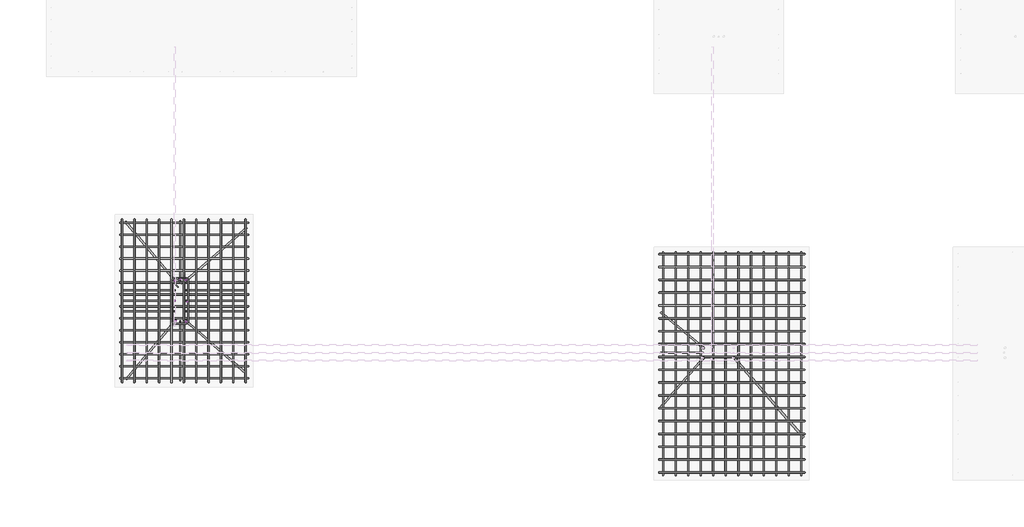
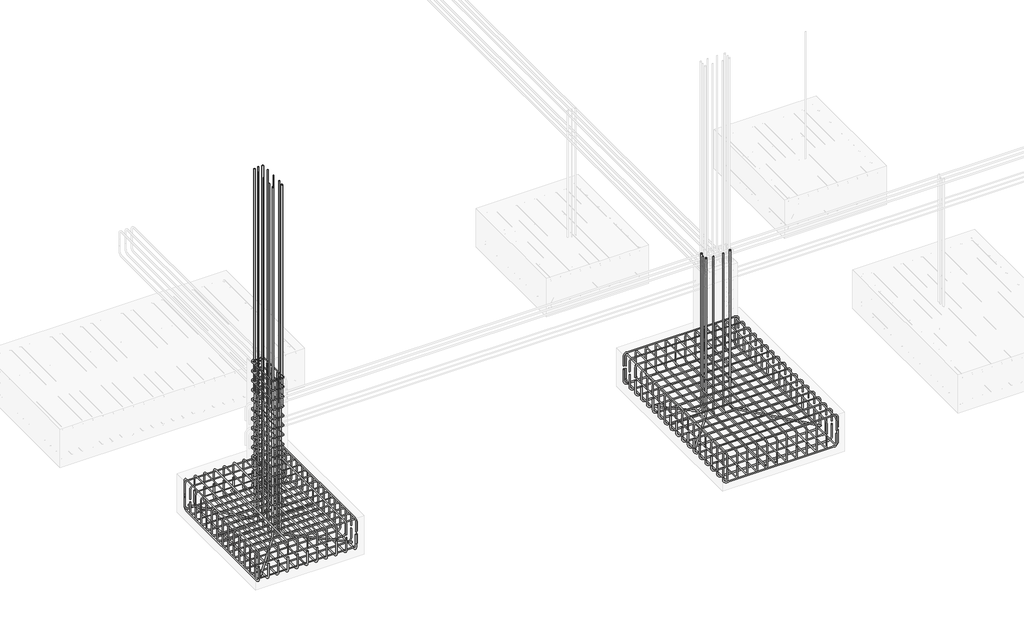
# One storey, part 2 of 18: 29 reinforcing bars.
"""IFC4 building model written with IfcOpenShell, lengths in millimetres."""

from ifc_helpers import new_model, si_unit, point, frame, origin, place, context, project, spatial, polyline, circle_curve, trimmed, segment, composite_curve, source, transform, mapped, element, save
from ifc_brep_helpers import swept_disk

model = new_model("IFC4")

# Units and contexts
model_context = context("Model", 3, world=origin())
ifc_project = project(units=[si_unit("LENGTHUNIT", "METRE", prefix="MILLI")], contexts=[model_context])

# Site, building, storey
site = spatial("IfcSite", under=ifc_project)
building = spatial("IfcBuilding", under=site)
storey = spatial("IfcBuildingStorey", under=building, Elevation=-2000.0)

# Reinforcing bars
placement = place(None, origin())
reinforcing_bar_shape = source(origin(), model_context, "Body", "SolidModel", [
    swept_disk(composite_curve([segment(polyline([(-15593.9747351, -4015.3521146, -2300.0), (-15593.9747351, -4015.3521146, -2486.6)]), True, "CONTINUOUS"), segment(trimmed(circle_curve(frame((-15593.9747351, -4070.8021146, -2486.6), z_axis=(-1.0, 0.0, 0.0), x_axis=(0.0, 55.45000000000027, 0.0)), 55.45), [point((-15593.9747351, -4015.3521146, -2486.6))], [point((-15593.9747351, -4070.8021146, -2542.05))], True, "CARTESIAN"), True, "CONTINUOUS"), segment(polyline([(-15593.9747351, -4070.8021146, -2542.05), (-15593.9747351, -5844.0021146, -2542.05)]), True, "CONTINUOUS"), segment(trimmed(circle_curve(frame((-15593.9747351, -5844.0021146, -2486.6), z_axis=(-1.0, 0.0, 0.0), x_axis=(0.0, 0.0, -55.45000000000027)), 55.45), [point((-15593.9747351, -5844.0021146, -2542.05))], [point((-15593.9747351, -5899.4521146, -2486.6))], True, "CARTESIAN"), True, "CONTINUOUS"), segment(polyline([(-15593.9747351, -5899.4521146, -2486.6), (-15593.9747351, -5899.4521146, -2300.0)]), True, "CONTINUOUS")], self_intersect=False), 7.95),
])
element("IfcReinforcingBar", 1, at=placement, inside=storey, context=model_context, shape_type="MappedRepresentation", body=[
    mapped(reinforcing_bar_shape, transform((0.0, 0.0, 0.0), x_axis=(1.0, 0.0, 0.0), y_axis=(0.0, 1.0, 0.0), z_axis=(0.0, 0.0, 1.0))),
    mapped(reinforcing_bar_shape, transform((143.267578, 0.0, 0.0), x_axis=(1.0, 0.0, 0.0), y_axis=(0.0, 1.0, 0.0), z_axis=(0.0, 0.0, 1.0))),
    mapped(reinforcing_bar_shape, transform((286.5351559, 0.0, 0.0), x_axis=(1.0, 0.0, 0.0), y_axis=(0.0, 1.0, 0.0), z_axis=(0.0, 0.0, 1.0))),
    mapped(reinforcing_bar_shape, transform((429.8027339, 0.0, 0.0), x_axis=(1.0, 0.0, 0.0), y_axis=(0.0, 1.0, 0.0), z_axis=(0.0, 0.0, 1.0))),
    mapped(reinforcing_bar_shape, transform((573.0703119, 0.0, 0.0), x_axis=(1.0, 0.0, 0.0), y_axis=(0.0, 1.0, 0.0), z_axis=(0.0, 0.0, 1.0))),
    mapped(reinforcing_bar_shape, transform((716.3378898, 0.0, 0.0), x_axis=(1.0, 0.0, 0.0), y_axis=(0.0, 1.0, 0.0), z_axis=(0.0, 0.0, 1.0))),
    mapped(reinforcing_bar_shape, transform((859.6054678, 0.0, 0.0), x_axis=(1.0, 0.0, 0.0), y_axis=(0.0, 1.0, 0.0), z_axis=(0.0, 0.0, 1.0))),
    mapped(reinforcing_bar_shape, transform((1002.8730457, 0.0, 0.0), x_axis=(1.0, 0.0, 0.0), y_axis=(0.0, 1.0, 0.0), z_axis=(0.0, 0.0, 1.0))),
    mapped(reinforcing_bar_shape, transform((1146.1406237, 0.0, 0.0), x_axis=(1.0, 0.0, 0.0), y_axis=(0.0, 1.0, 0.0), z_axis=(0.0, 0.0, 1.0))),
    mapped(reinforcing_bar_shape, transform((1289.4082017, 0.0, 0.0), x_axis=(1.0, 0.0, 0.0), y_axis=(0.0, 1.0, 0.0), z_axis=(0.0, 0.0, 1.0))),
    mapped(reinforcing_bar_shape, transform((1432.6757796, 0.0, 0.0), x_axis=(1.0, 0.0, 0.0), y_axis=(0.0, 1.0, 0.0), z_axis=(0.0, 0.0, 1.0))),
])
reinforcing_bar_2_shape = source(origin(), model_context, "Body", "SolidModel", [
    swept_disk(composite_curve([segment(polyline([(-15593.9747351, -5901.4021146, -2250.0), (-15593.9747351, -5901.4021146, -2102.0)]), True, "CONTINUOUS"), segment(trimmed(circle_curve(frame((-15593.9747351, -5855.4021146, -2102.0), z_axis=(-1.0, 0.0, 0.0), x_axis=(0.0, -46.0, 0.0)), 46.0), [point((-15593.9747351, -5901.4021146, -2102.0))], [point((-15593.9747351, -5855.4021146, -2056.0))], True, "CARTESIAN"), True, "CONTINUOUS"), segment(polyline([(-15593.9747351, -5855.4021146, -2056.0), (-15593.9747351, -4059.4021146, -2056.0)]), True, "CONTINUOUS"), segment(trimmed(circle_curve(frame((-15593.9747351, -4059.4021146, -2102.0), z_axis=(-1.0, 0.0, 0.0), x_axis=(0.0, 0.0, 46.0)), 46.0), [point((-15593.9747351, -4059.4021146, -2056.0))], [point((-15593.9747351, -4013.4021146, -2102.0))], True, "CARTESIAN"), True, "CONTINUOUS"), segment(polyline([(-15593.9747351, -4013.4021146, -2102.0), (-15593.9747351, -4013.4021146, -2250.0)]), True, "CONTINUOUS")], self_intersect=False), 6.0),
])
element("IfcReinforcingBar", 2, at=placement, inside=storey, context=model_context, shape_type="MappedRepresentation", body=[
    mapped(reinforcing_bar_2_shape, transform((0.0, 0.0, 0.0), x_axis=(1.0, 0.0, 0.0), y_axis=(0.0, 1.0, 0.0), z_axis=(0.0, 0.0, 1.0))),
    mapped(reinforcing_bar_2_shape, transform((143.267578, 0.0, 0.0), x_axis=(1.0, 0.0, 0.0), y_axis=(0.0, 1.0, 0.0), z_axis=(0.0, 0.0, 1.0))),
    mapped(reinforcing_bar_2_shape, transform((286.5351559, 0.0, 0.0), x_axis=(1.0, 0.0, 0.0), y_axis=(0.0, 1.0, 0.0), z_axis=(0.0, 0.0, 1.0))),
    mapped(reinforcing_bar_2_shape, transform((429.8027339, 0.0, 0.0), x_axis=(1.0, 0.0, 0.0), y_axis=(0.0, 1.0, 0.0), z_axis=(0.0, 0.0, 1.0))),
    mapped(reinforcing_bar_2_shape, transform((573.0703119, 0.0, 0.0), x_axis=(1.0, 0.0, 0.0), y_axis=(0.0, 1.0, 0.0), z_axis=(0.0, 0.0, 1.0))),
    mapped(reinforcing_bar_2_shape, transform((716.3378898, 0.0, 0.0), x_axis=(1.0, 0.0, 0.0), y_axis=(0.0, 1.0, 0.0), z_axis=(0.0, 0.0, 1.0))),
    mapped(reinforcing_bar_2_shape, transform((859.6054678, 0.0, 0.0), x_axis=(1.0, 0.0, 0.0), y_axis=(0.0, 1.0, 0.0), z_axis=(0.0, 0.0, 1.0))),
    mapped(reinforcing_bar_2_shape, transform((1002.8730457, 0.0, 0.0), x_axis=(1.0, 0.0, 0.0), y_axis=(0.0, 1.0, 0.0), z_axis=(0.0, 0.0, 1.0))),
    mapped(reinforcing_bar_2_shape, transform((1146.1406237, 0.0, 0.0), x_axis=(1.0, 0.0, 0.0), y_axis=(0.0, 1.0, 0.0), z_axis=(0.0, 0.0, 1.0))),
    mapped(reinforcing_bar_2_shape, transform((1289.4082017, 0.0, 0.0), x_axis=(1.0, 0.0, 0.0), y_axis=(0.0, 1.0, 0.0), z_axis=(0.0, 0.0, 1.0))),
    mapped(reinforcing_bar_2_shape, transform((1432.6757796, 0.0, 0.0), x_axis=(1.0, 0.0, 0.0), y_axis=(0.0, 1.0, 0.0), z_axis=(0.0, 0.0, 1.0))),
])
reinforcing_bar_3_shape = source(origin(), model_context, "Body", "SolidModel", [
    swept_disk(composite_curve([segment(polyline([(-15616.8702104, -5855.2213318, -2322.6684255), (-15616.8702104, -5855.2213318, -2470.6684255)]), True, "CONTINUOUS"), segment(trimmed(circle_curve(frame((-15570.8702104, -5855.2213318, -2470.6684255), z_axis=(0.0, -1.0, 0.0), x_axis=(-46.0, 0.0, 0.0)), 46.0), [point((-15616.8702104, -5855.2213318, -2470.6684255))], [point((-15570.8702104, -5855.2213318, -2516.6684255))], True, "CARTESIAN"), True, "CONTINUOUS"), segment(polyline([(-15570.8702104, -5855.2213318, -2516.6684255), (-14174.8702104, -5855.2213318, -2516.6684255)]), True, "CONTINUOUS"), segment(trimmed(circle_curve(frame((-14174.8702104, -5855.2213318, -2470.6684255), z_axis=(0.0, -1.0, 0.0), x_axis=(0.0, 0.0, -46.0)), 46.0), [point((-14174.8702104, -5855.2213318, -2516.6684255))], [point((-14128.8702104, -5855.2213318, -2470.6684255))], True, "CARTESIAN"), True, "CONTINUOUS"), segment(polyline([(-14128.8702104, -5855.2213318, -2470.6684255), (-14128.8702104, -5855.2213318, -2322.6684255)]), True, "CONTINUOUS")], self_intersect=False), 6.0),
])
element("IfcReinforcingBar", 3, at=placement, inside=storey, context=model_context, shape_type="MappedRepresentation", body=[
    mapped(reinforcing_bar_3_shape, transform((0.0, 0.0, 0.0), x_axis=(1.0, 0.0, 0.0), y_axis=(0.0, 1.0, 0.0), z_axis=(0.0, 0.0, 1.0))),
    mapped(reinforcing_bar_3_shape, transform((0.0, 138.7553125, 0.0), x_axis=(1.0, 0.0, 0.0), y_axis=(0.0, 1.0, 0.0), z_axis=(0.0, 0.0, 1.0))),
    mapped(reinforcing_bar_3_shape, transform((0.0, 277.510625, 0.0), x_axis=(1.0, 0.0, 0.0), y_axis=(0.0, 1.0, 0.0), z_axis=(0.0, 0.0, 1.0))),
    mapped(reinforcing_bar_3_shape, transform((0.0, 416.2659375, 0.0), x_axis=(1.0, 0.0, 0.0), y_axis=(0.0, 1.0, 0.0), z_axis=(0.0, 0.0, 1.0))),
    mapped(reinforcing_bar_3_shape, transform((0.0, 555.02125, 0.0), x_axis=(1.0, 0.0, 0.0), y_axis=(0.0, 1.0, 0.0), z_axis=(0.0, 0.0, 1.0))),
    mapped(reinforcing_bar_3_shape, transform((0.0, 693.7765624, 0.0), x_axis=(1.0, 0.0, 0.0), y_axis=(0.0, 1.0, 0.0), z_axis=(0.0, 0.0, 1.0))),
    mapped(reinforcing_bar_3_shape, transform((0.0, 832.5318749, 0.0), x_axis=(1.0, 0.0, 0.0), y_axis=(0.0, 1.0, 0.0), z_axis=(0.0, 0.0, 1.0))),
    mapped(reinforcing_bar_3_shape, transform((0.0, 971.2871874, 0.0), x_axis=(1.0, 0.0, 0.0), y_axis=(0.0, 1.0, 0.0), z_axis=(0.0, 0.0, 1.0))),
    mapped(reinforcing_bar_3_shape, transform((0.0, 1110.0424999, 0.0), x_axis=(1.0, 0.0, 0.0), y_axis=(0.0, 1.0, 0.0), z_axis=(0.0, 0.0, 1.0))),
    mapped(reinforcing_bar_3_shape, transform((0.0, 1248.7978124, 0.0), x_axis=(1.0, 0.0, 0.0), y_axis=(0.0, 1.0, 0.0), z_axis=(0.0, 0.0, 1.0))),
    mapped(reinforcing_bar_3_shape, transform((0.0, 1387.5531249, 0.0), x_axis=(1.0, 0.0, 0.0), y_axis=(0.0, 1.0, 0.0), z_axis=(0.0, 0.0, 1.0))),
    mapped(reinforcing_bar_3_shape, transform((0.0, 1526.3084374, 0.0), x_axis=(1.0, 0.0, 0.0), y_axis=(0.0, 1.0, 0.0), z_axis=(0.0, 0.0, 1.0))),
    mapped(reinforcing_bar_3_shape, transform((0.0, 1665.0637499, 0.0), x_axis=(1.0, 0.0, 0.0), y_axis=(0.0, 1.0, 0.0), z_axis=(0.0, 0.0, 1.0))),
    mapped(reinforcing_bar_3_shape, transform((0.0, 1803.8190623, 0.0), x_axis=(1.0, 0.0, 0.0), y_axis=(0.0, 1.0, 0.0), z_axis=(0.0, 0.0, 1.0))),
])
reinforcing_bar_4_shape = source(origin(), model_context, "Body", "SolidModel", [
    swept_disk(composite_curve([segment(polyline([(-15616.8702104, -4049.4790976, -2276.6677805), (-15616.8702104, -4049.4790976, -2128.6677805)]), True, "CONTINUOUS"), segment(trimmed(circle_curve(frame((-15570.8702104, -4049.4790976, -2128.6677805), z_axis=(0.0, 1.0, 0.0), x_axis=(-46.0, 0.0, 0.0)), 46.0), [point((-15616.8702104, -4049.4790976, -2128.6677805))], [point((-15570.8702104, -4049.4790976, -2082.6677805))], True, "CARTESIAN"), True, "CONTINUOUS"), segment(polyline([(-15570.8702104, -4049.4790976, -2082.6677805), (-14174.8702104, -4049.4790976, -2082.6677805)]), True, "CONTINUOUS"), segment(trimmed(circle_curve(frame((-14174.8702104, -4049.4790976, -2128.6677805), z_axis=(0.0, 1.0, 0.0), x_axis=(0.0, 0.0, 46.0)), 46.0), [point((-14174.8702104, -4049.4790976, -2082.6677805))], [point((-14128.8702104, -4049.4790976, -2128.6677805))], True, "CARTESIAN"), True, "CONTINUOUS"), segment(polyline([(-14128.8702104, -4049.4790976, -2128.6677805), (-14128.8702104, -4049.4790976, -2276.6677805)]), True, "CONTINUOUS")], self_intersect=False), 6.0),
])
element("IfcReinforcingBar", 4, at=placement, inside=storey, context=model_context, shape_type="MappedRepresentation", body=[
    mapped(reinforcing_bar_4_shape, transform((0.0, 0.0, 0.0), x_axis=(1.0, 0.0, 0.0), y_axis=(0.0, 1.0, 0.0), z_axis=(0.0, 0.0, 1.0))),
    mapped(reinforcing_bar_4_shape, transform((0.0, -138.9032488, 0.0), x_axis=(1.0, 0.0, 0.0), y_axis=(0.0, 1.0, 0.0), z_axis=(0.0, 0.0, 1.0))),
    mapped(reinforcing_bar_4_shape, transform((0.0, -277.8064976, 0.0), x_axis=(1.0, 0.0, 0.0), y_axis=(0.0, 1.0, 0.0), z_axis=(0.0, 0.0, 1.0))),
    mapped(reinforcing_bar_4_shape, transform((0.0, -416.7097463, 0.0), x_axis=(1.0, 0.0, 0.0), y_axis=(0.0, 1.0, 0.0), z_axis=(0.0, 0.0, 1.0))),
    mapped(reinforcing_bar_4_shape, transform((0.0, -555.6129951, 0.0), x_axis=(1.0, 0.0, 0.0), y_axis=(0.0, 1.0, 0.0), z_axis=(0.0, 0.0, 1.0))),
    mapped(reinforcing_bar_4_shape, transform((0.0, -694.5162439, 0.0), x_axis=(1.0, 0.0, 0.0), y_axis=(0.0, 1.0, 0.0), z_axis=(0.0, 0.0, 1.0))),
    mapped(reinforcing_bar_4_shape, transform((0.0, -833.4194927, 0.0), x_axis=(1.0, 0.0, 0.0), y_axis=(0.0, 1.0, 0.0), z_axis=(0.0, 0.0, 1.0))),
    mapped(reinforcing_bar_4_shape, transform((0.0, -972.3227415, 0.0), x_axis=(1.0, 0.0, 0.0), y_axis=(0.0, 1.0, 0.0), z_axis=(0.0, 0.0, 1.0))),
    mapped(reinforcing_bar_4_shape, transform((0.0, -1111.2259903, 0.0), x_axis=(1.0, 0.0, 0.0), y_axis=(0.0, 1.0, 0.0), z_axis=(0.0, 0.0, 1.0))),
    mapped(reinforcing_bar_4_shape, transform((0.0, -1250.129239, 0.0), x_axis=(1.0, 0.0, 0.0), y_axis=(0.0, 1.0, 0.0), z_axis=(0.0, 0.0, 1.0))),
    mapped(reinforcing_bar_4_shape, transform((0.0, -1389.0324878, 0.0), x_axis=(1.0, 0.0, 0.0), y_axis=(0.0, 1.0, 0.0), z_axis=(0.0, 0.0, 1.0))),
    mapped(reinforcing_bar_4_shape, transform((0.0, -1527.9357366, 0.0), x_axis=(1.0, 0.0, 0.0), y_axis=(0.0, 1.0, 0.0), z_axis=(0.0, 0.0, 1.0))),
    mapped(reinforcing_bar_4_shape, transform((0.0, -1666.8389854, 0.0), x_axis=(1.0, 0.0, 0.0), y_axis=(0.0, 1.0, 0.0), z_axis=(0.0, 0.0, 1.0))),
    mapped(reinforcing_bar_4_shape, transform((0.0, -1805.7422342, 0.0), x_axis=(1.0, 0.0, 0.0), y_axis=(0.0, 1.0, 0.0), z_axis=(0.0, 0.0, 1.0))),
])
reinforcing_bar_5_shape = source(origin(), model_context, "Body", "SolidModel", [
    swept_disk(composite_curve([segment(polyline([(-7678.5399692, -4415.5752408, -2300.0), (-7678.5399692, -4415.5752408, -2486.6)]), True, "CONTINUOUS"), segment(trimmed(circle_curve(frame((-7733.9899692, -4415.5752408, -2486.6), z_axis=(0.0, 1.0, 0.0), x_axis=(55.44999999999982, 0.0, 0.0)), 55.45), [point((-7678.5399692, -4415.5752408, -2486.6))], [point((-7733.9899692, -4415.5752408, -2542.05))], True, "CARTESIAN"), True, "CONTINUOUS"), segment(polyline([(-7733.9899692, -4415.5752408, -2542.05), (-9307.1899692, -4415.5752408, -2542.05)]), True, "CONTINUOUS"), segment(trimmed(circle_curve(frame((-9307.1899692, -4415.5752408, -2486.6), z_axis=(0.0, 1.0, 0.0), x_axis=(0.0, 0.0, -55.45000000000027)), 55.45), [point((-9307.1899692, -4415.5752408, -2542.05))], [point((-9362.6399692, -4415.5752408, -2486.6))], True, "CARTESIAN"), True, "CONTINUOUS"), segment(polyline([(-9362.6399692, -4415.5752408, -2486.6), (-9362.6399692, -4415.5752408, -2300.0)]), True, "CONTINUOUS")], self_intersect=False), 7.95),
])
element("IfcReinforcingBar", 5, at=placement, inside=storey, context=model_context, shape_type="MappedRepresentation", body=[
    mapped(reinforcing_bar_5_shape, transform((0.0, 0.0, 0.0), x_axis=(1.0, 0.0, 0.0), y_axis=(0.0, 1.0, 0.0), z_axis=(0.0, 0.0, 1.0))),
    mapped(reinforcing_bar_5_shape, transform((0.0, -148.9809282, 0.0), x_axis=(1.0, 0.0, 0.0), y_axis=(0.0, 1.0, 0.0), z_axis=(0.0, 0.0, 1.0))),
    mapped(reinforcing_bar_5_shape, transform((0.0, -297.9618564, 0.0), x_axis=(1.0, 0.0, 0.0), y_axis=(0.0, 1.0, 0.0), z_axis=(0.0, 0.0, 1.0))),
    mapped(reinforcing_bar_5_shape, transform((0.0, -446.9427846, 0.0), x_axis=(1.0, 0.0, 0.0), y_axis=(0.0, 1.0, 0.0), z_axis=(0.0, 0.0, 1.0))),
    mapped(reinforcing_bar_5_shape, transform((0.0, -595.9237129, 0.0), x_axis=(1.0, 0.0, 0.0), y_axis=(0.0, 1.0, 0.0), z_axis=(0.0, 0.0, 1.0))),
    mapped(reinforcing_bar_5_shape, transform((0.0, -744.9046411, 0.0), x_axis=(1.0, 0.0, 0.0), y_axis=(0.0, 1.0, 0.0), z_axis=(0.0, 0.0, 1.0))),
    mapped(reinforcing_bar_5_shape, transform((0.0, -893.8855693, 0.0), x_axis=(1.0, 0.0, 0.0), y_axis=(0.0, 1.0, 0.0), z_axis=(0.0, 0.0, 1.0))),
    mapped(reinforcing_bar_5_shape, transform((0.0, -1042.8664975, 0.0), x_axis=(1.0, 0.0, 0.0), y_axis=(0.0, 1.0, 0.0), z_axis=(0.0, 0.0, 1.0))),
    mapped(reinforcing_bar_5_shape, transform((0.0, -1191.8474257, 0.0), x_axis=(1.0, 0.0, 0.0), y_axis=(0.0, 1.0, 0.0), z_axis=(0.0, 0.0, 1.0))),
    mapped(reinforcing_bar_5_shape, transform((0.0, -1340.8283539, 0.0), x_axis=(1.0, 0.0, 0.0), y_axis=(0.0, 1.0, 0.0), z_axis=(0.0, 0.0, 1.0))),
    mapped(reinforcing_bar_5_shape, transform((0.0, -1489.8092821, 0.0), x_axis=(1.0, 0.0, 0.0), y_axis=(0.0, 1.0, 0.0), z_axis=(0.0, 0.0, 1.0))),
    mapped(reinforcing_bar_5_shape, transform((0.0, -1638.7902103, 0.0), x_axis=(1.0, 0.0, 0.0), y_axis=(0.0, 1.0, 0.0), z_axis=(0.0, 0.0, 1.0))),
    mapped(reinforcing_bar_5_shape, transform((0.0, -1787.7711386, 0.0), x_axis=(1.0, 0.0, 0.0), y_axis=(0.0, 1.0, 0.0), z_axis=(0.0, 0.0, 1.0))),
    mapped(reinforcing_bar_5_shape, transform((0.0, -1936.7520668, 0.0), x_axis=(1.0, 0.0, 0.0), y_axis=(0.0, 1.0, 0.0), z_axis=(0.0, 0.0, 1.0))),
    mapped(reinforcing_bar_5_shape, transform((0.0, -2085.732995, 0.0), x_axis=(1.0, 0.0, 0.0), y_axis=(0.0, 1.0, 0.0), z_axis=(0.0, 0.0, 1.0))),
    mapped(reinforcing_bar_5_shape, transform((0.0, -2234.7139232, 0.0), x_axis=(1.0, 0.0, 0.0), y_axis=(0.0, 1.0, 0.0), z_axis=(0.0, 0.0, 1.0))),
    mapped(reinforcing_bar_5_shape, transform((0.0, -2383.6948514, 0.0), x_axis=(1.0, 0.0, 0.0), y_axis=(0.0, 1.0, 0.0), z_axis=(0.0, 0.0, 1.0))),
    mapped(reinforcing_bar_5_shape, transform((0.0, -2532.6757796, 0.0), x_axis=(1.0, 0.0, 0.0), y_axis=(0.0, 1.0, 0.0), z_axis=(0.0, 0.0, 1.0))),
])
reinforcing_bar_6_shape = source(origin(), model_context, "Body", "SolidModel", [
    swept_disk(composite_curve([segment(polyline([(-9364.5899692, -4415.5752408, -2250.0), (-9364.5899692, -4415.5752408, -2102.0)]), True, "CONTINUOUS"), segment(trimmed(circle_curve(frame((-9318.5899692, -4415.5752408, -2102.0), z_axis=(0.0, 1.0, 0.0), x_axis=(-46.0, 0.0, 0.0)), 46.0), [point((-9364.5899692, -4415.5752408, -2102.0))], [point((-9318.5899692, -4415.5752408, -2056.0))], True, "CARTESIAN"), True, "CONTINUOUS"), segment(polyline([(-9318.5899692, -4415.5752408, -2056.0), (-7722.5899692, -4415.5752408, -2056.0)]), True, "CONTINUOUS"), segment(trimmed(circle_curve(frame((-7722.5899692, -4415.5752408, -2102.0), z_axis=(0.0, 1.0, 0.0), x_axis=(0.0, 0.0, 46.0)), 46.0), [point((-7722.5899692, -4415.5752408, -2056.0))], [point((-7676.5899692, -4415.5752408, -2102.0))], True, "CARTESIAN"), True, "CONTINUOUS"), segment(polyline([(-7676.5899692, -4415.5752408, -2102.0), (-7676.5899692, -4415.5752408, -2250.0)]), True, "CONTINUOUS")], self_intersect=False), 6.0),
])
element("IfcReinforcingBar", 6, at=placement, inside=storey, context=model_context, shape_type="MappedRepresentation", body=[
    mapped(reinforcing_bar_6_shape, transform((0.0, 0.0, 0.0), x_axis=(1.0, 0.0, 0.0), y_axis=(0.0, 1.0, 0.0), z_axis=(0.0, 0.0, 1.0))),
    mapped(reinforcing_bar_6_shape, transform((0.0, -148.9809282, 0.0), x_axis=(1.0, 0.0, 0.0), y_axis=(0.0, 1.0, 0.0), z_axis=(0.0, 0.0, 1.0))),
    mapped(reinforcing_bar_6_shape, transform((0.0, -297.9618564, 0.0), x_axis=(1.0, 0.0, 0.0), y_axis=(0.0, 1.0, 0.0), z_axis=(0.0, 0.0, 1.0))),
    mapped(reinforcing_bar_6_shape, transform((0.0, -446.9427846, 0.0), x_axis=(1.0, 0.0, 0.0), y_axis=(0.0, 1.0, 0.0), z_axis=(0.0, 0.0, 1.0))),
    mapped(reinforcing_bar_6_shape, transform((0.0, -595.9237129, 0.0), x_axis=(1.0, 0.0, 0.0), y_axis=(0.0, 1.0, 0.0), z_axis=(0.0, 0.0, 1.0))),
    mapped(reinforcing_bar_6_shape, transform((0.0, -744.9046411, 0.0), x_axis=(1.0, 0.0, 0.0), y_axis=(0.0, 1.0, 0.0), z_axis=(0.0, 0.0, 1.0))),
    mapped(reinforcing_bar_6_shape, transform((0.0, -893.8855693, 0.0), x_axis=(1.0, 0.0, 0.0), y_axis=(0.0, 1.0, 0.0), z_axis=(0.0, 0.0, 1.0))),
    mapped(reinforcing_bar_6_shape, transform((0.0, -1042.8664975, 0.0), x_axis=(1.0, 0.0, 0.0), y_axis=(0.0, 1.0, 0.0), z_axis=(0.0, 0.0, 1.0))),
    mapped(reinforcing_bar_6_shape, transform((0.0, -1191.8474257, 0.0), x_axis=(1.0, 0.0, 0.0), y_axis=(0.0, 1.0, 0.0), z_axis=(0.0, 0.0, 1.0))),
    mapped(reinforcing_bar_6_shape, transform((0.0, -1340.8283539, 0.0), x_axis=(1.0, 0.0, 0.0), y_axis=(0.0, 1.0, 0.0), z_axis=(0.0, 0.0, 1.0))),
    mapped(reinforcing_bar_6_shape, transform((0.0, -1489.8092821, 0.0), x_axis=(1.0, 0.0, 0.0), y_axis=(0.0, 1.0, 0.0), z_axis=(0.0, 0.0, 1.0))),
    mapped(reinforcing_bar_6_shape, transform((0.0, -1638.7902103, 0.0), x_axis=(1.0, 0.0, 0.0), y_axis=(0.0, 1.0, 0.0), z_axis=(0.0, 0.0, 1.0))),
    mapped(reinforcing_bar_6_shape, transform((0.0, -1787.7711386, 0.0), x_axis=(1.0, 0.0, 0.0), y_axis=(0.0, 1.0, 0.0), z_axis=(0.0, 0.0, 1.0))),
    mapped(reinforcing_bar_6_shape, transform((0.0, -1936.7520668, 0.0), x_axis=(1.0, 0.0, 0.0), y_axis=(0.0, 1.0, 0.0), z_axis=(0.0, 0.0, 1.0))),
    mapped(reinforcing_bar_6_shape, transform((0.0, -2085.732995, 0.0), x_axis=(1.0, 0.0, 0.0), y_axis=(0.0, 1.0, 0.0), z_axis=(0.0, 0.0, 1.0))),
    mapped(reinforcing_bar_6_shape, transform((0.0, -2234.7139232, 0.0), x_axis=(1.0, 0.0, 0.0), y_axis=(0.0, 1.0, 0.0), z_axis=(0.0, 0.0, 1.0))),
    mapped(reinforcing_bar_6_shape, transform((0.0, -2383.6948514, 0.0), x_axis=(1.0, 0.0, 0.0), y_axis=(0.0, 1.0, 0.0), z_axis=(0.0, 0.0, 1.0))),
    mapped(reinforcing_bar_6_shape, transform((0.0, -2532.6757796, 0.0), x_axis=(1.0, 0.0, 0.0), y_axis=(0.0, 1.0, 0.0), z_axis=(0.0, 0.0, 1.0))),
])
reinforcing_bar_7_shape = source(origin(), model_context, "Body", "SolidModel", [
    swept_disk(composite_curve([segment(polyline([(-9318.4091864, -4392.6797656, -2322.6684255), (-9318.4091864, -4392.6797656, -2470.6684255)]), True, "CONTINUOUS"), segment(trimmed(circle_curve(frame((-9318.4091864, -4438.6797656, -2470.6684255), z_axis=(-1.0, 0.0, 0.0), x_axis=(0.0, 46.0, 0.0)), 46.0), [point((-9318.4091864, -4392.6797656, -2470.6684255))], [point((-9318.4091864, -4438.6797656, -2516.6684255))], True, "CARTESIAN"), True, "CONTINUOUS"), segment(polyline([(-9318.4091864, -4438.6797656, -2516.6684255), (-9318.4091864, -6934.6797656, -2516.6684255)]), True, "CONTINUOUS"), segment(trimmed(circle_curve(frame((-9318.4091864, -6934.6797656, -2470.6684255), z_axis=(-1.0, 0.0, 0.0), x_axis=(0.0, 0.0, -46.0)), 46.0), [point((-9318.4091864, -6934.6797656, -2516.6684255))], [point((-9318.4091864, -6980.6797656, -2470.6684255))], True, "CARTESIAN"), True, "CONTINUOUS"), segment(polyline([(-9318.4091864, -6980.6797656, -2470.6684255), (-9318.4091864, -6980.6797656, -2322.6684255)]), True, "CONTINUOUS")], self_intersect=False), 6.0),
])
element("IfcReinforcingBar", 7, at=placement, inside=storey, context=model_context, shape_type="MappedRepresentation", body=[
    mapped(reinforcing_bar_7_shape, transform((0.0, 0.0, 0.0), x_axis=(1.0, 0.0, 0.0), y_axis=(0.0, 1.0, 0.0), z_axis=(0.0, 0.0, 1.0))),
    mapped(reinforcing_bar_7_shape, transform((145.8017329, 0.0, 0.0), x_axis=(1.0, 0.0, 0.0), y_axis=(0.0, 1.0, 0.0), z_axis=(0.0, 0.0, 1.0))),
    mapped(reinforcing_bar_7_shape, transform((291.6034659, 0.0, 0.0), x_axis=(1.0, 0.0, 0.0), y_axis=(0.0, 1.0, 0.0), z_axis=(0.0, 0.0, 1.0))),
    mapped(reinforcing_bar_7_shape, transform((437.4051988, 0.0, 0.0), x_axis=(1.0, 0.0, 0.0), y_axis=(0.0, 1.0, 0.0), z_axis=(0.0, 0.0, 1.0))),
    mapped(reinforcing_bar_7_shape, transform((583.2069318, 0.0, 0.0), x_axis=(1.0, 0.0, 0.0), y_axis=(0.0, 1.0, 0.0), z_axis=(0.0, 0.0, 1.0))),
    mapped(reinforcing_bar_7_shape, transform((729.0086647, 0.0, 0.0), x_axis=(1.0, 0.0, 0.0), y_axis=(0.0, 1.0, 0.0), z_axis=(0.0, 0.0, 1.0))),
    mapped(reinforcing_bar_7_shape, transform((874.8103976, 0.0, 0.0), x_axis=(1.0, 0.0, 0.0), y_axis=(0.0, 1.0, 0.0), z_axis=(0.0, 0.0, 1.0))),
    mapped(reinforcing_bar_7_shape, transform((1020.6121306, 0.0, 0.0), x_axis=(1.0, 0.0, 0.0), y_axis=(0.0, 1.0, 0.0), z_axis=(0.0, 0.0, 1.0))),
    mapped(reinforcing_bar_7_shape, transform((1166.4138635, 0.0, 0.0), x_axis=(1.0, 0.0, 0.0), y_axis=(0.0, 1.0, 0.0), z_axis=(0.0, 0.0, 1.0))),
    mapped(reinforcing_bar_7_shape, transform((1312.2155965, 0.0, 0.0), x_axis=(1.0, 0.0, 0.0), y_axis=(0.0, 1.0, 0.0), z_axis=(0.0, 0.0, 1.0))),
    mapped(reinforcing_bar_7_shape, transform((1458.0173294, 0.0, 0.0), x_axis=(1.0, 0.0, 0.0), y_axis=(0.0, 1.0, 0.0), z_axis=(0.0, 0.0, 1.0))),
    mapped(reinforcing_bar_7_shape, transform((1603.8190623, 0.0, 0.0), x_axis=(1.0, 0.0, 0.0), y_axis=(0.0, 1.0, 0.0), z_axis=(0.0, 0.0, 1.0))),
])
reinforcing_bar_8_shape = source(origin(), model_context, "Body", "SolidModel", [
    swept_disk(composite_curve([segment(polyline([(-7712.6669522, -4392.6797656, -2276.6677805), (-7712.6669522, -4392.6797656, -2128.6677805)]), True, "CONTINUOUS"), segment(trimmed(circle_curve(frame((-7712.6669522, -4438.6797656, -2128.6677805), z_axis=(1.0, 0.0, 0.0), x_axis=(0.0, 46.0, 0.0)), 46.0), [point((-7712.6669522, -4392.6797656, -2128.6677805))], [point((-7712.6669522, -4438.6797656, -2082.6677805))], True, "CARTESIAN"), True, "CONTINUOUS"), segment(polyline([(-7712.6669522, -4438.6797656, -2082.6677805), (-7712.6669522, -6934.6797656, -2082.6677805)]), True, "CONTINUOUS"), segment(trimmed(circle_curve(frame((-7712.6669522, -6934.6797656, -2128.6677805), z_axis=(1.0, 0.0, 0.0), x_axis=(0.0, 0.0, 46.0)), 46.0), [point((-7712.6669522, -6934.6797656, -2082.6677805))], [point((-7712.6669522, -6980.6797656, -2128.6677805))], True, "CARTESIAN"), True, "CONTINUOUS"), segment(polyline([(-7712.6669522, -6980.6797656, -2128.6677805), (-7712.6669522, -6980.6797656, -2276.6677805)]), True, "CONTINUOUS")], self_intersect=False), 6.0),
])
element("IfcReinforcingBar", 8, at=placement, inside=storey, context=model_context, shape_type="MappedRepresentation", body=[
    mapped(reinforcing_bar_8_shape, transform((0.0, 0.0, 0.0), x_axis=(1.0, 0.0, 0.0), y_axis=(0.0, 1.0, 0.0), z_axis=(0.0, 0.0, 1.0))),
    mapped(reinforcing_bar_8_shape, transform((-145.9765667, 0.0, 0.0), x_axis=(1.0, 0.0, 0.0), y_axis=(0.0, 1.0, 0.0), z_axis=(0.0, 0.0, 1.0))),
    mapped(reinforcing_bar_8_shape, transform((-291.9531335, 0.0, 0.0), x_axis=(1.0, 0.0, 0.0), y_axis=(0.0, 1.0, 0.0), z_axis=(0.0, 0.0, 1.0))),
    mapped(reinforcing_bar_8_shape, transform((-437.9297002, 0.0, 0.0), x_axis=(1.0, 0.0, 0.0), y_axis=(0.0, 1.0, 0.0), z_axis=(0.0, 0.0, 1.0))),
    mapped(reinforcing_bar_8_shape, transform((-583.906267, 0.0, 0.0), x_axis=(1.0, 0.0, 0.0), y_axis=(0.0, 1.0, 0.0), z_axis=(0.0, 0.0, 1.0))),
    mapped(reinforcing_bar_8_shape, transform((-729.8828337, 0.0, 0.0), x_axis=(1.0, 0.0, 0.0), y_axis=(0.0, 1.0, 0.0), z_axis=(0.0, 0.0, 1.0))),
    mapped(reinforcing_bar_8_shape, transform((-875.8594005, 0.0, 0.0), x_axis=(1.0, 0.0, 0.0), y_axis=(0.0, 1.0, 0.0), z_axis=(0.0, 0.0, 1.0))),
    mapped(reinforcing_bar_8_shape, transform((-1021.8359672, 0.0, 0.0), x_axis=(1.0, 0.0, 0.0), y_axis=(0.0, 1.0, 0.0), z_axis=(0.0, 0.0, 1.0))),
    mapped(reinforcing_bar_8_shape, transform((-1167.8125339, 0.0, 0.0), x_axis=(1.0, 0.0, 0.0), y_axis=(0.0, 1.0, 0.0), z_axis=(0.0, 0.0, 1.0))),
    mapped(reinforcing_bar_8_shape, transform((-1313.7891007, 0.0, 0.0), x_axis=(1.0, 0.0, 0.0), y_axis=(0.0, 1.0, 0.0), z_axis=(0.0, 0.0, 1.0))),
    mapped(reinforcing_bar_8_shape, transform((-1459.7656674, 0.0, 0.0), x_axis=(1.0, 0.0, 0.0), y_axis=(0.0, 1.0, 0.0), z_axis=(0.0, 0.0, 1.0))),
    mapped(reinforcing_bar_8_shape, transform((-1605.7422342, 0.0, 0.0), x_axis=(1.0, 0.0, 0.0), y_axis=(0.0, 1.0, 0.0), z_axis=(0.0, 0.0, 1.0))),
])
element("IfcReinforcingBar", 9, at=placement, inside=storey, context=model_context, shape_type="SolidModel", body=[
    swept_disk(composite_curve([segment(polyline([(-9343.8693064, -5088.6530082, -2480.0), (-8900.4558049, -5460.7211138, -2480.0)]), True, "CONTINUOUS"), segment(trimmed(circle_curve(frame((-8900.4558049, -5460.7211138, -2412.5), z_axis=(-0.6427876096865429, -0.7660444431189751, 0.0), x_axis=(0.0, 0.0, -67.5)), 67.5), [point((-8900.4558049, -5460.7211138, -2480.0))], [point((-8848.747805, -5504.1092774, -2412.5))], True, "CARTESIAN"), True, "CONTINUOUS"), segment(polyline([(-8848.747805, -5504.1092774, -2412.5), (-8848.747805, -5504.1092774, -20.0)]), True, "CONTINUOUS")], self_intersect=False), 10.0),
])
element("IfcReinforcingBar", 10, at=placement, inside=storey, context=model_context, shape_type="SolidModel", body=[
    swept_disk(composite_curve([segment(polyline([(-9347.9036256, -5559.3632831, -2480.0), (-8905.107931, -5559.3632831, -2480.0)]), True, "CONTINUOUS"), segment(trimmed(circle_curve(frame((-8905.107931, -5559.3632831, -2434.0), z_axis=(0.0, -1.0, 0.0), x_axis=(0.0, 0.0, -46.0)), 46.0), [point((-8905.107931, -5559.3632831, -2480.0))], [point((-8859.107931, -5559.3632831, -2434.0))], True, "CARTESIAN"), True, "CONTINUOUS"), segment(polyline([(-8859.107931, -5559.3632831, -2434.0), (-8859.107931, -5559.3632831, -30.0)]), True, "CONTINUOUS")], self_intersect=False), 6.0),
])
element("IfcReinforcingBar", 11, at=placement, inside=storey, context=model_context, shape_type="SolidModel", body=[
    swept_disk(composite_curve([segment(polyline([(-9350.8701529, -6196.8759393, -2480.0), (-8893.0317894, -5670.1931504, -2480.0)]), True, "CONTINUOUS"), segment(trimmed(circle_curve(frame((-8893.0317894, -5670.1931504, -2412.5), z_axis=(0.7547095802227678, -0.6560590289905122, 0.0), x_axis=(0.0, 0.0, -67.5)), 67.5), [point((-8893.0317894, -5670.1931504, -2480.0))], [point((-8848.747805, -5619.2502537, -2412.5))], True, "CARTESIAN"), True, "CONTINUOUS"), segment(polyline([(-8848.747805, -5619.2502537, -2412.5), (-8848.747805, -5619.2502537, -20.0)]), True, "CONTINUOUS")], self_intersect=False), 10.0),
])
element("IfcReinforcingBar", 12, at=placement, inside=storey, context=model_context, shape_type="SolidModel", body=[
    swept_disk(composite_curve([segment(polyline([(-7690.3097855, -6541.9864615, -2480.0), (-8448.148149, -5670.1931504, -2480.0)]), True, "CONTINUOUS"), segment(trimmed(circle_curve(frame((-8448.148149, -5670.1931504, -2412.5), z_axis=(0.7547095802227678, 0.6560590289905122, 0.0), x_axis=(0.0, 0.0, -67.5)), 67.5), [point((-8448.148149, -5670.1931504, -2480.0))], [point((-8492.4321335, -5619.2502537, -2412.5))], True, "CARTESIAN"), True, "CONTINUOUS"), segment(polyline([(-8492.4321335, -5619.2502537, -2412.5), (-8492.4321335, -5619.2502537, -20.0)]), True, "CONTINUOUS")], self_intersect=False), 10.0),
])
reinforcing_bar_9_shape = source(origin(), model_context, "Body", "SolidModel", [
    swept_disk(composite_curve([segment(polyline([(-8743.6420643, -6948.2510204, -2480.0), (-8743.6420643, -5673.717598, -2480.0)]), True, "CONTINUOUS"), segment(trimmed(circle_curve(frame((-8743.6420643, -5673.717598, -2434.0), z_axis=(1.0, 0.0, 0.0), x_axis=(0.0, 0.0, -46.0)), 46.0), [point((-8743.6420643, -5673.717598, -2480.0))], [point((-8743.6420643, -5627.717598, -2434.0))], True, "CARTESIAN"), True, "CONTINUOUS"), segment(polyline([(-8743.6420643, -5627.717598, -2434.0), (-8743.6420643, -5627.717598, -30.0)]), True, "CONTINUOUS")], self_intersect=False), 6.0),
])
element("IfcReinforcingBar", 13, at=placement, inside=storey, context=model_context, shape_type="MappedRepresentation", body=[
    mapped(reinforcing_bar_9_shape, transform((0.0, 0.0, 0.0), x_axis=(1.0, 0.0, 0.0), y_axis=(0.0, 1.0, 0.0), z_axis=(0.0, 0.0, 1.0))),
    mapped(reinforcing_bar_9_shape, transform((144.9594019, 0.0, 0.0), x_axis=(1.0, 0.0, 0.0), y_axis=(0.0, 1.0, 0.0), z_axis=(0.0, 0.0, 1.0))),
])
reinforcing_bar_10_shape = source(origin(), model_context, "Body", "SolidModel", [
    swept_disk(composite_curve([segment(polyline([(-14944.0408553, -4797.2436629, -34.0), (-15000.376307, -4740.9082112, -34.0)]), True, "CONTINUOUS"), segment(trimmed(circle_curve(frame((-14979.8702104, -4720.4021146, -34.0), z_axis=(0.0, 0.0, -1.0), x_axis=(-20.50609660000009, -20.50609660000009, 0.0)), 29.0), [point((-15000.376307, -4740.9082112, -34.0))], [point((-14979.8702104, -4691.4021146, -34.0))], True, "CARTESIAN"), True, "CONTINUOUS"), segment(polyline([(-14979.8702104, -4691.4021146, -34.0), (-14855.8702104, -4691.4021146, -34.0)]), True, "CONTINUOUS"), segment(trimmed(circle_curve(frame((-14855.8702104, -4720.4021146, -34.0), z_axis=(0.0, 0.0, -1.0), x_axis=(0.0, 29.0, 0.0)), 29.0), [point((-14855.8702104, -4691.4021146, -34.0))], [point((-14826.8702104, -4720.4021146, -34.0))], True, "CARTESIAN"), True, "CONTINUOUS"), segment(polyline([(-14826.8702104, -4720.4021146, -34.0), (-14826.8702104, -5194.4021146, -34.0)]), True, "CONTINUOUS"), segment(trimmed(circle_curve(frame((-14855.8422349, -5194.4021146, -32.7265044), z_axis=(-0.04391364091329579, 0.0, -0.9990353307775147), x_axis=(28.972024499998952, 0.0, -1.2734955999999968)), 29.0), [point((-14826.8702104, -5194.4021146, -34.0))], [point((-14855.8422349, -5223.4021146, -32.7265044))], True, "CARTESIAN"), True, "CONTINUOUS"), segment(polyline([(-14855.8422349, -5223.4021146, -32.7265044), (-14979.8981858, -5223.4021146, -27.2734956)]), True, "CONTINUOUS"), segment(trimmed(circle_curve(frame((-14979.8981858, -5194.4021146, -27.2734956), z_axis=(-0.04391364091329579, 0.0, -0.9990353307775147), x_axis=(0.0, -29.0, 0.0)), 29.0), [point((-14979.8981858, -5223.4021146, -27.2734956))], [point((-15008.8702104, -5194.4021146, -26.0))], True, "CARTESIAN"), True, "CONTINUOUS"), segment(polyline([(-15008.8702104, -5194.4021146, -26.0), (-15008.8702104, -4720.4021146, -26.0)]), True, "CONTINUOUS"), segment(trimmed(circle_curve(frame((-14979.8702104, -4720.4021146, -26.0), z_axis=(0.0, 0.0, -1.0), x_axis=(-29.0, 0.0, 0.0)), 29.0), [point((-15008.8702104, -4720.4021146, -26.0))], [point((-14959.3641137, -4699.8960179, -26.0))], True, "CARTESIAN"), True, "CONTINUOUS"), segment(polyline([(-14959.3641137, -4699.8960179, -26.0), (-14903.028662, -4756.2314696, -26.0)]), True, "CONTINUOUS")], self_intersect=False), 4.0),
])
element("IfcReinforcingBar", 14, at=placement, inside=storey, context=model_context, shape_type="MappedRepresentation", body=[
    mapped(reinforcing_bar_10_shape, transform((0.0, 0.0, 0.0), x_axis=(1.0, 0.0, 0.0), y_axis=(0.0, 1.0, 0.0), z_axis=(0.0, 0.0, 1.0))),
    mapped(reinforcing_bar_10_shape, transform((0.0, 0.0, -148.6153846), x_axis=(1.0, 0.0, 0.0), y_axis=(0.0, 1.0, 0.0), z_axis=(0.0, 0.0, 1.0))),
    mapped(reinforcing_bar_10_shape, transform((0.0, 0.0, -297.2307692), x_axis=(1.0, 0.0, 0.0), y_axis=(0.0, 1.0, 0.0), z_axis=(0.0, 0.0, 1.0))),
    mapped(reinforcing_bar_10_shape, transform((0.0, 0.0, -445.8461538), x_axis=(1.0, 0.0, 0.0), y_axis=(0.0, 1.0, 0.0), z_axis=(0.0, 0.0, 1.0))),
    mapped(reinforcing_bar_10_shape, transform((0.0, 0.0, -594.4615385), x_axis=(1.0, 0.0, 0.0), y_axis=(0.0, 1.0, 0.0), z_axis=(0.0, 0.0, 1.0))),
    mapped(reinforcing_bar_10_shape, transform((0.0, 0.0, -743.0769231), x_axis=(1.0, 0.0, 0.0), y_axis=(0.0, 1.0, 0.0), z_axis=(0.0, 0.0, 1.0))),
    mapped(reinforcing_bar_10_shape, transform((0.0, 0.0, -891.6923077), x_axis=(1.0, 0.0, 0.0), y_axis=(0.0, 1.0, 0.0), z_axis=(0.0, 0.0, 1.0))),
    mapped(reinforcing_bar_10_shape, transform((0.0, 0.0, -1040.3076923), x_axis=(1.0, 0.0, 0.0), y_axis=(0.0, 1.0, 0.0), z_axis=(0.0, 0.0, 1.0))),
    mapped(reinforcing_bar_10_shape, transform((0.0, 0.0, -1188.9230769), x_axis=(1.0, 0.0, 0.0), y_axis=(0.0, 1.0, 0.0), z_axis=(0.0, 0.0, 1.0))),
    mapped(reinforcing_bar_10_shape, transform((0.0, 0.0, -1337.5384615), x_axis=(1.0, 0.0, 0.0), y_axis=(0.0, 1.0, 0.0), z_axis=(0.0, 0.0, 1.0))),
    mapped(reinforcing_bar_10_shape, transform((0.0, 0.0, -1486.1538462), x_axis=(1.0, 0.0, 0.0), y_axis=(0.0, 1.0, 0.0), z_axis=(0.0, 0.0, 1.0))),
    mapped(reinforcing_bar_10_shape, transform((0.0, 0.0, -1634.7692308), x_axis=(1.0, 0.0, 0.0), y_axis=(0.0, 1.0, 0.0), z_axis=(0.0, 0.0, 1.0))),
    mapped(reinforcing_bar_10_shape, transform((0.0, 0.0, -1783.3846154), x_axis=(1.0, 0.0, 0.0), y_axis=(0.0, 1.0, 0.0), z_axis=(0.0, 0.0, 1.0))),
    mapped(reinforcing_bar_10_shape, transform((0.0, 0.0, -1932.0), x_axis=(1.0, 0.0, 0.0), y_axis=(0.0, 1.0, 0.0), z_axis=(0.0, 0.0, 1.0))),
])
element("IfcReinforcingBar", 15, at=placement, inside=storey, context=model_context, shape_type="SolidModel", body=[
    swept_disk(composite_curve([segment(polyline([(-15545.7670007, -5865.24837, -2480.0), (-15018.8288622, -5237.2679502, -2480.0)]), True, "CONTINUOUS"), segment(trimmed(circle_curve(frame((-15018.8288622, -5237.2679502, -2412.5), z_axis=(0.7660444431189727, -0.6427876096865457, 0.0), x_axis=(0.0, 0.0, -67.5)), 67.5), [point((-15018.8288622, -5237.2679502, -2480.0))], [point((-14975.4406985, -5185.5599503, -2412.5))], True, "CARTESIAN"), True, "CONTINUOUS"), segment(polyline([(-14975.4406985, -5185.5599503, -2412.5), (-14975.4406985, -5185.5599503, -30.0)]), True, "CONTINUOUS")], self_intersect=False), 10.0),
])
element("IfcReinforcingBar", 16, at=placement, inside=storey, context=model_context, shape_type="SolidModel", body=[
    swept_disk(composite_curve([segment(polyline([(-14920.1866928, -5884.715771, -2480.0), (-14920.1866928, -5241.9200764, -2480.0)]), True, "CONTINUOUS"), segment(trimmed(circle_curve(frame((-14920.1866928, -5241.9200764, -2434.0), z_axis=(1.0, 0.0, 0.0), x_axis=(0.0, 0.0, -46.0)), 46.0), [point((-14920.1866928, -5241.9200764, -2480.0))], [point((-14920.1866928, -5195.9200764, -2434.0))], True, "CARTESIAN"), True, "CONTINUOUS"), segment(polyline([(-14920.1866928, -5195.9200764, -2434.0), (-14920.1866928, -5195.9200764, -30.0)]), True, "CONTINUOUS")], self_intersect=False), 6.0),
])
element("IfcReinforcingBar", 17, at=placement, inside=storey, context=model_context, shape_type="SolidModel", body=[
    swept_disk(composite_curve([segment(polyline([(-15553.8850345, -4039.8811633, -2480.0), (-15018.8288622, -4677.5362789, -2480.0)]), True, "CONTINUOUS"), segment(trimmed(circle_curve(frame((-15018.8288622, -4677.5362789, -2412.5), z_axis=(-0.7660444431189773, -0.6427876096865401, 0.0), x_axis=(0.0, 0.0, -67.5)), 67.5), [point((-15018.8288622, -4677.5362789, -2480.0))], [point((-14975.4406985, -4729.2442788, -2412.5))], True, "CARTESIAN"), True, "CONTINUOUS"), segment(polyline([(-14975.4406985, -4729.2442788, -2412.5), (-14975.4406985, -4729.2442788, -30.0)]), True, "CONTINUOUS")], self_intersect=False), 10.0),
])
element("IfcReinforcingBar", 18, at=placement, inside=storey, context=model_context, shape_type="SolidModel", body=[
    swept_disk(composite_curve([segment(polyline([(-14158.0253025, -5796.0377897, -2480.0), (-14809.3568255, -5229.8439348, -2480.0)]), True, "CONTINUOUS"), segment(trimmed(circle_curve(frame((-14809.3568255, -5229.8439348, -2412.5), z_axis=(0.6560590289905148, 0.7547095802227656, 0.0), x_axis=(0.0, 0.0, -67.5)), 67.5), [point((-14809.3568255, -5229.8439348, -2480.0))], [point((-14860.2997222, -5185.5599503, -2412.5))], True, "CARTESIAN"), True, "CONTINUOUS"), segment(polyline([(-14860.2997222, -5185.5599503, -2412.5), (-14860.2997222, -5185.5599503, -30.0)]), True, "CONTINUOUS")], self_intersect=False), 10.0),
])
element("IfcReinforcingBar", 19, at=placement, inside=storey, context=model_context, shape_type="SolidModel", body=[
    swept_disk(composite_curve([segment(polyline([(-14147.9050181, -4109.9690105, -2480.0), (-14809.3568255, -4684.9602944, -2480.0)]), True, "CONTINUOUS"), segment(trimmed(circle_curve(frame((-14809.3568255, -4684.9602944, -2412.5), z_axis=(-0.6560590289905096, 0.75470958022277, 0.0), x_axis=(0.0, 0.0, -67.5)), 67.5), [point((-14809.3568255, -4684.9602944, -2480.0))], [point((-14860.2997222, -4729.2442788, -2412.5))], True, "CARTESIAN"), True, "CONTINUOUS"), segment(polyline([(-14860.2997222, -4729.2442788, -2412.5), (-14860.2997222, -4729.2442788, -30.0)]), True, "CONTINUOUS")], self_intersect=False), 10.0),
])
element("IfcReinforcingBar", 20, at=placement, inside=storey, context=model_context, shape_type="SolidModel", body=[
    swept_disk(composite_curve([segment(polyline([(-14920.1866928, -4030.0884582, -2480.0), (-14920.1866928, -4672.8841528, -2480.0)]), True, "CONTINUOUS"), segment(trimmed(circle_curve(frame((-14920.1866928, -4672.8841528, -2434.0), z_axis=(-1.0, 0.0, 0.0), x_axis=(0.0, 0.0, -46.0)), 46.0), [point((-14920.1866928, -4672.8841528, -2480.0))], [point((-14920.1866928, -4718.8841528, -2434.0))], True, "CARTESIAN"), True, "CONTINUOUS"), segment(polyline([(-14920.1866928, -4718.8841528, -2434.0), (-14920.1866928, -4718.8841528, -30.0)]), True, "CONTINUOUS")], self_intersect=False), 6.0),
])
reinforcing_bar_11_shape = source(origin(), model_context, "Body", "SolidModel", [
    swept_disk(composite_curve([segment(polyline([(-14161.2989555, -5080.4542096, -2480.0), (-14805.8323779, -5080.4542096, -2480.0)]), True, "CONTINUOUS"), segment(trimmed(circle_curve(frame((-14805.8323779, -5080.4542096, -2434.0), z_axis=(0.0, 1.0, 0.0), x_axis=(0.0, 0.0, -46.0)), 46.0), [point((-14805.8323779, -5080.4542096, -2480.0))], [point((-14851.8323779, -5080.4542096, -2434.0))], True, "CARTESIAN"), True, "CONTINUOUS"), segment(polyline([(-14851.8323779, -5080.4542096, -2434.0), (-14851.8323779, -5080.4542096, -30.0)]), True, "CONTINUOUS")], self_intersect=False), 6.0),
])
element("IfcReinforcingBar", 21, at=placement, inside=storey, context=model_context, shape_type="MappedRepresentation", body=[
    mapped(reinforcing_bar_11_shape, transform((0.0, 0.0, 0.0), x_axis=(1.0, 0.0, 0.0), y_axis=(0.0, 1.0, 0.0), z_axis=(0.0, 0.0, 1.0))),
    mapped(reinforcing_bar_11_shape, transform((0.0, 122.4797009, 0.0), x_axis=(1.0, 0.0, 0.0), y_axis=(0.0, 1.0, 0.0), z_axis=(0.0, 0.0, 1.0))),
    mapped(reinforcing_bar_11_shape, transform((0.0, 244.9594019, 0.0), x_axis=(1.0, 0.0, 0.0), y_axis=(0.0, 1.0, 0.0), z_axis=(0.0, 0.0, 1.0))),
])
reinforcing_bar_12_shape = source(origin(), model_context, "Body", "SolidModel", [
    swept_disk(composite_curve([segment(polyline([(-15592.9156249, -5080.4542096, -2480.0), (-15029.9080428, -5080.4542096, -2480.0)]), True, "CONTINUOUS"), segment(trimmed(circle_curve(frame((-15029.9080428, -5080.4542096, -2434.0), z_axis=(0.0, -1.0, 0.0), x_axis=(0.0, 0.0, -46.0)), 46.0), [point((-15029.9080428, -5080.4542096, -2480.0))], [point((-14983.9080428, -5080.4542096, -2434.0))], True, "CARTESIAN"), True, "CONTINUOUS"), segment(polyline([(-14983.9080428, -5080.4542096, -2434.0), (-14983.9080428, -5080.4542096, -30.0)]), True, "CONTINUOUS")], self_intersect=False), 6.0),
])
element("IfcReinforcingBar", 22, at=placement, inside=storey, context=model_context, shape_type="MappedRepresentation", body=[
    mapped(reinforcing_bar_12_shape, transform((0.0, 0.0, 0.0), x_axis=(1.0, 0.0, 0.0), y_axis=(0.0, 1.0, 0.0), z_axis=(0.0, 0.0, 1.0))),
    mapped(reinforcing_bar_12_shape, transform((0.0, 122.4797009, 0.0), x_axis=(1.0, 0.0, 0.0), y_axis=(0.0, 1.0, 0.0), z_axis=(0.0, 0.0, 1.0))),
    mapped(reinforcing_bar_12_shape, transform((0.0, 244.9594019, 0.0), x_axis=(1.0, 0.0, 0.0), y_axis=(0.0, 1.0, 0.0), z_axis=(0.0, 0.0, 1.0))),
])
element("IfcReinforcingBar", 23, at=placement, inside=storey, context=model_context, shape_type="SolidModel", body=[
    swept_disk(composite_curve([segment(polyline([(-14976.7205241, -4724.9138218, -480.0), (-14976.7205241, -4724.9138218, 2970.0)]), True, "CONTINUOUS")], self_intersect=False), 10.0),
])
element("IfcReinforcingBar", 24, at=placement, inside=storey, context=model_context, shape_type="SolidModel", body=[
    swept_disk(composite_curve([segment(polyline([(-14851.5795478, -4714.9138218, -480.0), (-14851.5795478, -4714.9138218, 2970.0)]), True, "CONTINUOUS")], self_intersect=False), 10.0),
])
reinforcing_bar_13_shape = source(origin(), model_context, "Body", "SolidModel", [
    swept_disk(composite_curve([segment(polyline([(-14838.872385, -5109.4403335, -480.0), (-14838.872385, -5109.4403335, 2970.0)]), True, "CONTINUOUS")], self_intersect=False), 6.0),
])
element("IfcReinforcingBar", 25, at=placement, inside=storey, context=model_context, shape_type="MappedRepresentation", body=[
    mapped(reinforcing_bar_13_shape, transform((0.0, 0.0, 0.0), x_axis=(1.0, 0.0, 0.0), y_axis=(0.0, 1.0, 0.0), z_axis=(0.0, 0.0, 1.0))),
    mapped(reinforcing_bar_13_shape, transform((0.0, 141.3852466, 0.0), x_axis=(1.0, 0.0, 0.0), y_axis=(0.0, 1.0, 0.0), z_axis=(0.0, 0.0, 1.0))),
    mapped(reinforcing_bar_13_shape, transform((0.0, 282.7704933, 0.0), x_axis=(1.0, 0.0, 0.0), y_axis=(0.0, 1.0, 0.0), z_axis=(0.0, 0.0, 1.0))),
])
reinforcing_bar_14_shape = source(origin(), model_context, "Body", "SolidModel", [
    swept_disk(composite_curve([segment(polyline([(-14980.1878684, -5099.4403335, -480.0), (-14980.1878684, -5099.4403335, 2970.0)]), True, "CONTINUOUS")], self_intersect=False), 6.0),
])
element("IfcReinforcingBar", 26, at=placement, inside=storey, context=model_context, shape_type="MappedRepresentation", body=[
    mapped(reinforcing_bar_14_shape, transform((0.0, 0.0, 0.0), x_axis=(1.0, 0.0, 0.0), y_axis=(0.0, 1.0, 0.0), z_axis=(0.0, 0.0, 1.0))),
    mapped(reinforcing_bar_14_shape, transform((0.0, 141.3852466, 0.0), x_axis=(1.0, 0.0, 0.0), y_axis=(0.0, 1.0, 0.0), z_axis=(0.0, 0.0, 1.0))),
    mapped(reinforcing_bar_14_shape, transform((0.0, 282.7704933, 0.0), x_axis=(1.0, 0.0, 0.0), y_axis=(0.0, 1.0, 0.0), z_axis=(0.0, 0.0, 1.0))),
])
element("IfcReinforcingBar", 27, at=placement, inside=storey, context=model_context, shape_type="SolidModel", body=[
    swept_disk(composite_curve([segment(polyline([(-14916.4665184, -4709.5536958, -480.0), (-14916.4665184, -4709.5536958, 2970.0)]), True, "CONTINUOUS")], self_intersect=False), 6.0),
])
element("IfcReinforcingBar", 28, at=placement, inside=storey, context=model_context, shape_type="SolidModel", body=[
    swept_disk(composite_curve([segment(polyline([(-14976.7205241, -5189.8904074, -480.0), (-14976.7205241, -5189.8904074, 2970.0)]), True, "CONTINUOUS")], self_intersect=False), 10.0),
])
element("IfcReinforcingBar", 29, at=placement, inside=storey, context=model_context, shape_type="SolidModel", body=[
    swept_disk(composite_curve([segment(polyline([(-14851.5795478, -5199.8904074, -480.0), (-14851.5795478, -5199.8904074, 2970.0)]), True, "CONTINUOUS")], self_intersect=False), 10.0),
])

save(model, "model.ifc")

# Revit data of these elements
# Elements 1, 2, 3, 4, 5, 6, 7, 8, 9, 10, 11, 12, 13, 14, 15, 16, 17, 18, 19, 20, 21, 22, 23, 24, 25, 26, 27, 28, 29 (IfcReinforcingBar)
#   Phase Created = New Construction
